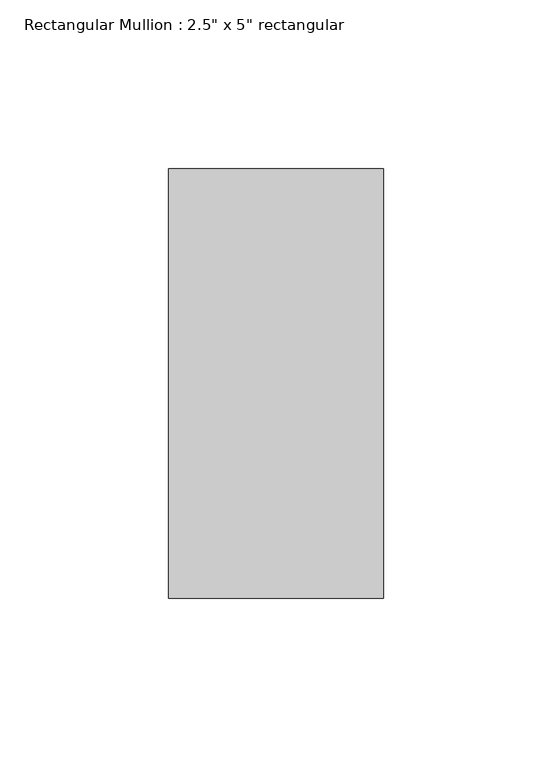
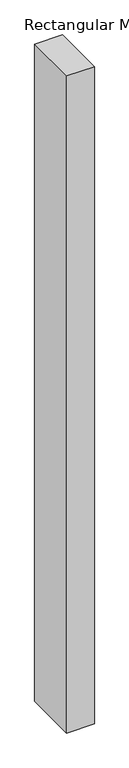
"""IFC4 building model written with IfcOpenShell, lengths in millimetres: member geometry."""

from ifc_helpers import new_model, si_unit, frame, origin, place, context, project, spatial, polyline, outline, extrude, source, transform, mapped, element, save


def member_cb82b20f(model_context):
    return source(origin(), model_context, "Body", "SweptSolid", [
        extrude(outline(polyline([(31.75, 63.5), (31.75, -63.5), (-31.75, -63.5), (-31.75, 63.5), (31.75, 63.5)])), frame((0.0, 0.0, -1594.6445261), z_axis=(0.0, 0.0, 1.0), x_axis=(1.0, 0.0, 0.0)), (0.0, 0.0, 1.0), 1594.6445261),
    ])


if __name__ == "__main__":
    model = new_model("IFC4")
    model_context = context("Model", 3, world=origin())
    ifc_project = project(units=[si_unit("LENGTHUNIT", "METRE", prefix="MILLI")], contexts=[model_context])
    site = spatial("IfcSite", under=ifc_project)
    building = spatial("IfcBuilding", under=site)
    placement = place(None, origin())
    member_shape = member_cb82b20f(model_context)
    element("IfcMember", 1, ObjectType="Rectangular Mullion : 2.5\" x 5\" rectangular", at=placement, inside=building, context=model_context, shape_type="MappedRepresentation", body=[
        mapped(member_shape, transform((0.0, 0.0, 0.0), x_axis=(1.0, 0.0, 0.0), y_axis=(0.0, 1.0, 0.0), z_axis=(0.0, 0.0, 1.0))),
    ])
    save(model, "model.ifc")

# Revit data of these elements
# Type "Rectangular Mullion : 2.5\" x 5\" rectangular"
#   built-in parameter 1007304 = 0.416667 (stored number, unit not read)
#   built-in parameter 1007301 = 0.104167 (stored number, unit not read)
#   built-in parameter 1007300 = 0.104167 (stored number, unit not read)
# Element 1 (IfcMember, "Rectangular Mullion : 2.5\" x 5\" rectangular")
#   Materials on its faces: "Aluminum"
# Materials
#   "Aluminum": class "Metal", colour RGB 247 247 247, transparency 0, Description = "Aluminum 6061", Cost = 0
